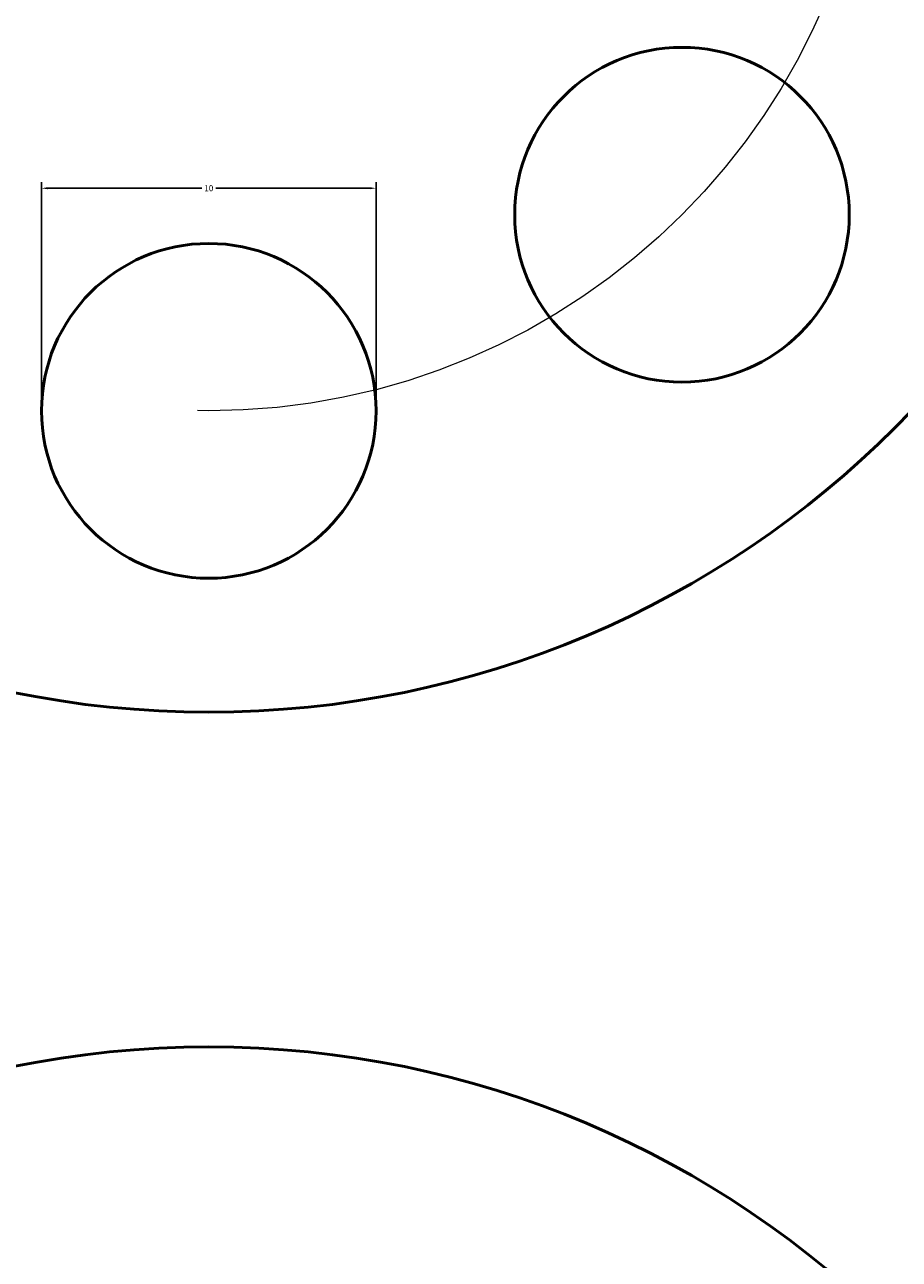
# Model space of a CAD drawing. Units: inches. Extents: x -11 to 126, y -62 to 82.
# Tile 8 of 10: x 54 to 80, y 1 to 38. Entities that reach past the tile are written whole.
import ezdxf

# ---------------------------------------------------------------- set-up
doc = ezdxf.new("R2010")
doc.units = ezdxf.units.IN
doc.header["$MEASUREMENT"] = 0
doc.linetypes.add('CENTER', pattern=[50.8, 31.75, -6.35, 6.35, -6.35])
for name, color, linetype, lineweight in [('M-CNTR', 4, 'CENTER', 18), ('M-DIMS', 2, 'Continuous', 18), ('M-OUTL', 7, 'Continuous', 50)]:
    doc.layers.add(name, color=color, linetype=linetype, lineweight=lineweight)
doc.styles.get("Standard").update_dxf_attribs({"font": 'arial.ttf'})
doc.dimstyles.get("Standard").update_dxf_attribs({"dimtxt": 0.18, "dimasz": 0.18, "dimexe": 0.18, "dimexo": 0.0625, "dimgap": 0.09, "dimtad": 0, "dimtih": 1, "dimtoh": 1, "dimdec": 4, "dimzin": 0, "dimdsep": 46, "dimtxsty": 'Standard', "dimcen": 0.09, "dimadec": 0, "dimazin": 0, "dimtfac": 1, "dimtdec": 4, "dimtofl": 0, "dimtmove": 0, "dimatfit": 3, "dimfxl": 1, "dimtolj": 1, "dimtzin": 0, "dimarcsym": 0})

# ---------------------------------------------------------------- blocks, each defined once
blk = doc.blocks.new('*U1')
blk.add_circle((0, 0), 5)
blk = doc.blocks.new('*U2')
at = {"layer": 'M-OUTL', "color": 0, "linetype": 'ByBlock', "lineweight": -2, "transparency": 16777216, "rotation": 44.99999999999998}
blk.add_blockref('*U1', (73.374, 32.212), dxfattribs=at)
at = {"layer": 'M-OUTL', "color": 0, "linetype": 'ByBlock', "lineweight": -2, "transparency": 16777216}
blk.add_blockref('*U1', (59.232, 26.354), dxfattribs=at)
blk = doc.blocks.new('*D5')
at = {"layer": 'Defpoints', "color": 0, "transparency": 16777216}
for p in [(119.232, 12.354), (-0.749, 11.479), (119.232, -57.296)]:
    blk.add_point(p, dxfattribs=at)
at = {"layer": 'M-DIMS', "color": 0, "lineweight": -2, "transparency": 16777216}
for p, q in [((119.232, 12.292), (119.232, -57.476)), ((-0.749, 11.416), (-0.749, -57.476)), ((-0.569, -57.296), (58.786, -57.296)), ((119.052, -57.296), (59.696, -57.296))]:
    blk.add_line(p, q, dxfattribs=at)
at = {"layer": 'M-DIMS', "color": 0, "transparency": 16777216}
for points in [[(-0.569, -57.266), (-0.569, -57.326), (-0.749, -57.296)], [(119.052, -57.266), (119.052, -57.326), (119.232, -57.296)]]:
    blk.add_solid(points, dxfattribs=at)
at = {"layer": 'M-DIMS', "color": 0, "transparency": 16777216, "insert": (59.241, -57.296), "char_height": 0.18, "attachment_point": 5}
blk.add_mtext('\\A1;119.98', dxfattribs=at)
blk = doc.blocks.new('*D6')
at = {"layer": 'Defpoints', "color": 0, "transparency": 16777216}
for p in [(-7.399, 75.354), (59.232, 75.354), (59.232, -50.646)]:
    blk.add_point(p, dxfattribs=at)
at = {"layer": 'M-DIMS', "color": 0, "lineweight": -2, "transparency": 16777216}
for p, q in [((59.169, 75.354), (-7.579, 75.354)), ((-7.399, 75.174), (-7.399, 12.536)), ((-7.399, -50.466), (-7.399, 12.172)), ((59.169, -50.646), (-7.579, -50.646))]:
    blk.add_line(p, q, dxfattribs=at)
at = {"layer": 'M-DIMS', "color": 0, "transparency": 16777216}
for points in [[(-7.429, 75.174), (-7.369, 75.174), (-7.399, 75.354)], [(-7.429, -50.466), (-7.369, -50.466), (-7.399, -50.646)]]:
    blk.add_solid(points, dxfattribs=at)
at = {"layer": 'M-DIMS', "color": 0, "transparency": 16777216, "insert": (-7.399, 12.354), "char_height": 0.18, "attachment_point": 5}
blk.add_mtext('\\A1;126', dxfattribs=at)
blk = doc.blocks.new('*D7')
at = {"layer": 'Defpoints', "color": 0, "transparency": 16777216}
for p in [(59.232, 82.004), (59.232, 46.354), (19.232, 12.354)]:
    blk.add_point(p, dxfattribs=at)
at = {"layer": 'M-DIMS', "color": 0, "lineweight": -2, "transparency": 16777216}
for p, q in [((19.232, 12.417), (19.232, 82.184)), ((19.412, 82.004), (39.009, 82.004)), ((59.052, 82.004), (39.454, 82.004)), ((59.232, 46.417), (59.232, 82.184))]:
    blk.add_line(p, q, dxfattribs=at)
at = {"layer": 'M-DIMS', "color": 0, "transparency": 16777216}
for points in [[(19.412, 82.034), (19.412, 81.974), (19.232, 82.004)], [(59.052, 82.034), (59.052, 81.974), (59.232, 82.004)]]:
    blk.add_solid(points, dxfattribs=at)
at = {"layer": 'M-DIMS', "color": 0, "transparency": 16777216, "insert": (39.232, 82.004), "char_height": 0.18, "attachment_point": 5}
blk.add_mtext('\\A1;40', dxfattribs=at)
blk = doc.blocks.new('*D8')
at = {"layer": 'Defpoints', "color": 0, "transparency": 16777216}
for p in [(99.232, 82.004), (59.232, 46.354), (99.232, 12.354)]:
    blk.add_point(p, dxfattribs=at)
at = {"layer": 'M-DIMS', "color": 0, "lineweight": -2, "transparency": 16777216}
for p, q in [((59.232, 46.417), (59.232, 82.184)), ((59.412, 82.004), (79.009, 82.004)), ((99.052, 82.004), (79.454, 82.004)), ((99.232, 12.417), (99.232, 82.184))]:
    blk.add_line(p, q, dxfattribs=at)
at = {"layer": 'M-DIMS', "color": 0, "transparency": 16777216}
for points in [[(59.412, 82.034), (59.412, 81.974), (59.232, 82.004)], [(99.052, 82.034), (99.052, 81.974), (99.232, 82.004)]]:
    blk.add_solid(points, dxfattribs=at)
at = {"layer": 'M-DIMS', "color": 0, "transparency": 16777216, "insert": (79.232, 82.004), "char_height": 0.18, "attachment_point": 5}
blk.add_mtext('\\A1;40', dxfattribs=at)
blk = doc.blocks.new('*D9')
at = {"layer": 'Defpoints', "color": 0, "transparency": 16777216}
for p in [(99.232, 12.354), (125.882, 12.354), (59.232, -21.646)]:
    blk.add_point(p, dxfattribs=at)
at = {"layer": 'M-DIMS', "color": 0, "lineweight": -2, "transparency": 16777216}
for p, q in [((99.294, 12.354), (126.062, 12.354)), ((125.882, 12.174), (125.882, -4.464)), ((125.882, -21.466), (125.882, -4.828)), ((59.294, -21.646), (126.062, -21.646))]:
    blk.add_line(p, q, dxfattribs=at)
at = {"layer": 'M-DIMS', "color": 0, "transparency": 16777216}
for points in [[(125.852, 12.174), (125.912, 12.174), (125.882, 12.354)], [(125.852, -21.466), (125.912, -21.466), (125.882, -21.646)]]:
    blk.add_solid(points, dxfattribs=at)
at = {"layer": 'M-DIMS', "color": 0, "transparency": 16777216, "insert": (125.882, -4.646), "char_height": 0.18, "attachment_point": 5}
blk.add_mtext('\\A1;34', dxfattribs=at)
blk = doc.blocks.new('*D10')
at = {"layer": 'Defpoints', "color": 0, "transparency": 16777216}
for p in [(59.232, 46.354), (125.882, 46.354), (99.232, 12.354)]:
    blk.add_point(p, dxfattribs=at)
at = {"layer": 'M-DIMS', "color": 0, "lineweight": -2, "transparency": 16777216}
for p, q in [((59.294, 46.354), (126.062, 46.354)), ((125.882, 46.174), (125.882, 29.536)), ((125.882, 12.534), (125.882, 29.172)), ((99.294, 12.354), (126.062, 12.354))]:
    blk.add_line(p, q, dxfattribs=at)
at = {"layer": 'M-DIMS', "color": 0, "transparency": 16777216}
for points in [[(125.852, 46.174), (125.912, 46.174), (125.882, 46.354)], [(125.852, 12.534), (125.912, 12.534), (125.882, 12.354)]]:
    blk.add_solid(points, dxfattribs=at)
at = {"layer": 'M-DIMS', "color": 0, "transparency": 16777216, "insert": (125.882, 29.354), "char_height": 0.18, "attachment_point": 5}
blk.add_mtext('\\A1;34', dxfattribs=at)
blk = doc.blocks.new('*D11')
at = {"layer": 'Defpoints', "color": 0, "transparency": 16777216}
for p in [(64.232, 33.004), (54.232, 26.354), (64.232, 26.354)]:
    blk.add_point(p, dxfattribs=at)
at = {"layer": 'M-DIMS', "color": 0, "lineweight": -2, "transparency": 16777216}
for p, q in [((54.232, 26.417), (54.232, 33.184)), ((54.412, 33.004), (59.021, 33.004)), ((64.052, 33.004), (59.442, 33.004)), ((64.232, 26.417), (64.232, 33.184))]:
    blk.add_line(p, q, dxfattribs=at)
at = {"layer": 'M-DIMS', "color": 0, "transparency": 16777216}
for points in [[(54.412, 33.034), (54.412, 32.974), (54.232, 33.004)], [(64.052, 33.034), (64.052, 32.974), (64.232, 33.004)]]:
    blk.add_solid(points, dxfattribs=at)
at = {"layer": 'M-DIMS', "color": 0, "transparency": 16777216, "insert": (59.232, 33.004), "char_height": 0.18, "attachment_point": 5}
blk.add_mtext('\\A1;10', dxfattribs=at)
blk = doc.blocks.new('*D13')
at = {"layer": 'Defpoints', "color": 0, "transparency": 16777216}
for p in [(73.731, 3.469), (44.732, -46.761)]:
    blk.add_point(p, dxfattribs=at)
at = {"layer": 'M-DIMS', "color": 0, "lineweight": -2, "transparency": 16777216}
for p, q in [((59.142, -21.646), (59.322, -21.646)), ((59.232, -21.736), (59.232, -21.556)), ((36.032, -61.83), (44.642, -46.917)), ((35.852, -61.83), (36.032, -61.83))]:
    blk.add_line(p, q, dxfattribs=at)
at = {"layer": 'M-DIMS', "color": 0, "transparency": 16777216}
blk.add_solid([(44.616, -46.902), (44.668, -46.932), (44.732, -46.761)], dxfattribs=at)
at = {"layer": 'M-DIMS', "color": 0, "transparency": 16777216, "insert": (35.345, -61.83), "char_height": 0.18, "attachment_point": 5}
blk.add_mtext('\\A1;2X ∅58', dxfattribs=at)

msp = doc.modelspace()

# ---------------------------------------------------------------- linework, layer by layer
at = {"layer": 'M-CNTR'}
msp.add_circle((59.232, 46.354), 20, dxfattribs=at)
at = {"layer": 'M-OUTL'}
for centre in [(59.232, 46.354), (59.232, -21.646)]:
    msp.add_circle(centre, 29, dxfattribs=at)

# ---------------------------------------------------------------- block references
msp.add_blockref('*U2', (0, 0), dxfattribs=at)

# ---------------------------------------------------------------- dimensions: what is measured, and where the dimension line sits
at = {"layer": 'M-DIMS'}
for base, p1, p2, override, picture, middle in [((59.232, 82.004), (19.232, 12.354), (59.232, 46.354), {"dimdec": 0, "dimlfac": 1, "dimrnd": 0, "dimzin": 0, "dimdsep": 46, "dimlunit": 2}, '*D7', (39.232, 82.004)), ((99.232, 82.004), (59.232, 46.354), (99.232, 12.354), {"dimdec": 0, "dimlfac": 1, "dimrnd": 0, "dimzin": 0, "dimdsep": 46, "dimlunit": 2}, '*D8', (79.232, 82.004)), ((64.232, 33.004), (54.232, 26.354), (64.232, 26.354), {"dimdec": 0, "dimlfac": 1, "dimrnd": 0, "dimzin": 0, "dimdsep": 46, "dimlunit": 2}, '*D11', (59.232, 33.004)), ((119.232, -57.296), (-0.749, 11.479), (119.232, 12.354), {"dimdec": 2, "dimlfac": 1, "dimrnd": 0, "dimzin": 0, "dimdsep": 46, "dimlunit": 2}, '*D5', (59.241, -57.296))]:
    dim = msp.add_linear_dim(base=base, p1=p1, p2=p2, dimstyle='Standard', override=override, dxfattribs=at)
    dim.commit()
    dim.dimension.update_dxf_attribs({"geometry": picture, "text_midpoint": middle})
for base, p1, p2, picture, middle in [((-7.399, 75.354), (59.232, -50.646), (59.232, 75.354), '*D6', (-7.399, 12.354)), ((125.882, 46.354), (99.232, 12.354), (59.232, 46.354), '*D10', (125.882, 29.354)), ((125.882, 12.354), (59.232, -21.646), (99.232, 12.354), '*D9', (125.882, -4.646))]:
    dim = msp.add_linear_dim(base=base, p1=p1, p2=p2, angle=90, dimstyle='Standard', override={"dimdec": 0, "dimlfac": 1, "dimrnd": 0, "dimzin": 0, "dimdsep": 46, "dimlunit": 2}, dxfattribs=at)
    dim.commit()
    dim.dimension.update_dxf_attribs({"geometry": picture, "text_midpoint": middle})
dim = msp.add_diameter_dim_2p(p1=(73.731, 3.469), p2=(44.732, -46.761), text='2X <>', dimstyle='Standard', override={"dimdec": 0, "dimlfac": 1, "dimrnd": 0, "dimzin": 0, "dimdsep": 46, "dimlunit": 2}, dxfattribs=at)
dim.commit()
dim.dimension.update_dxf_attribs({"geometry": '*D13', "text_midpoint": (35.345, -61.83), "dimtype": 163})

doc.saveas('drawing.dxf')
